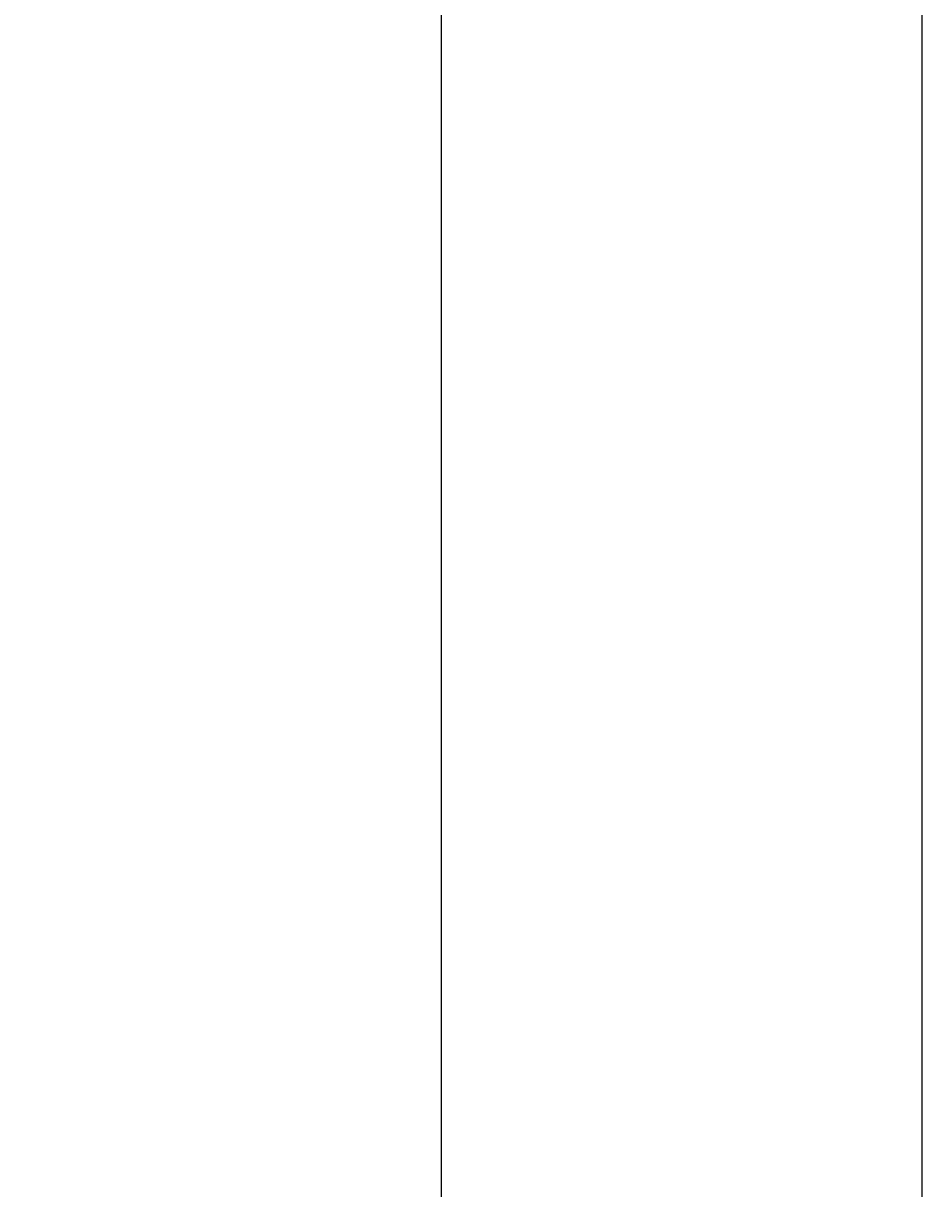
# Model space of a CAD drawing. Units: inches. Extents: x 738 to 1068, y 378 to 757.
# Tile 15 of 41: x 911 to 939, y 399 to 435. Entities that reach past the tile are written whole.
import ezdxf

# ---------------------------------------------------------------- set-up
doc = ezdxf.new("R2010")
doc.units = ezdxf.units.IN
doc.header["$MEASUREMENT"] = 0
doc.layers.add('A-ANNO-DIMS', color=2, linetype='Continuous', lineweight=18)
doc.styles.get("Standard").update_dxf_attribs({"font": 'arial.ttf'})
doc.dimstyles.get("Standard").update_dxf_attribs({"dimtxt": 0.18, "dimasz": 0.18, "dimexe": 0.18, "dimexo": 0.0625, "dimgap": 0.09, "dimtad": 0, "dimtih": 1, "dimtoh": 1, "dimdec": 4, "dimzin": 0, "dimdsep": 46, "dimtxsty": 'Standard', "dimcen": 0.09, "dimadec": 0, "dimazin": 0, "dimtfac": 1, "dimtdec": 4, "dimtofl": 0, "dimtmove": 0, "dimatfit": 3, "dimfxl": 1, "dimtolj": 1, "dimtzin": 0, "dimarcsym": 0})

# ---------------------------------------------------------------- blocks, each defined once
blk = doc.blocks.new('*D17')
at = {"layer": 'A-ANNO-DIMS', "color": 0, "lineweight": -2, "transparency": 16777216}
for p, q in [((756.324, 415.842), (756.324, 378.239)), ((1050.049, 415.919), (1050.049, 378.239)), ((756.504, 378.419), (902.791, 378.419)), ((1049.869, 378.419), (903.582, 378.419))]:
    blk.add_line(p, q, dxfattribs=at)
at = {"layer": 'A-ANNO-DIMS', "color": 0, "transparency": 16777216}
for points in [[(756.504, 378.449), (756.504, 378.389), (756.324, 378.419)], [(1049.869, 378.449), (1049.869, 378.389), (1050.049, 378.419)]]:
    blk.add_solid(points, dxfattribs=at)
at = {"layer": 'Defpoints', "color": 0, "transparency": 16777216}
for p in [(756.324, 415.904), (1050.049, 415.982), (1050.049, 378.419)]:
    blk.add_point(p, dxfattribs=at)
at = {"layer": 'A-ANNO-DIMS', "color": 0, "transparency": 16777216, "insert": (903.186, 378.419), "char_height": 0.18, "attachment_point": 5}
blk.add_mtext('\\A1;293.7', dxfattribs=at)
blk = doc.blocks.new('*D18')
at = {"layer": 'A-ANNO-DIMS', "color": 0, "lineweight": -2, "transparency": 16777216}
for p, q in [((901.525, 738.375), (1068.179, 738.375)), ((1067.999, 738.195), (1067.999, 569.167)), ((1067.999, 399.775), (1067.999, 568.803)), ((1023.842, 399.595), (1068.179, 399.595))]:
    blk.add_line(p, q, dxfattribs=at)
at = {"layer": 'A-ANNO-DIMS', "color": 0, "transparency": 16777216}
for points in [[(1067.969, 738.195), (1068.029, 738.195), (1067.999, 738.375)], [(1067.969, 399.775), (1068.029, 399.775), (1067.999, 399.595)]]:
    blk.add_solid(points, dxfattribs=at)
at = {"layer": 'Defpoints', "color": 0, "transparency": 16777216}
for p in [(901.462, 738.375), (1067.999, 738.375), (1023.779, 399.595)]:
    blk.add_point(p, dxfattribs=at)
at = {"layer": 'A-ANNO-DIMS', "color": 0, "transparency": 16777216, "insert": (1067.999, 568.985), "char_height": 0.18, "attachment_point": 5}
blk.add_mtext('\\A1;338.8', dxfattribs=at)
blk = doc.blocks.new('*D27')
at = {"layer": 'A-ANNO-DIMS', "color": 0, "lineweight": -2, "transparency": 16777216}
for p, q in [((883.457, 646.923), (883.457, 378.239)), ((923.511, 646.923), (923.511, 378.239)), ((883.637, 378.419), (903.086, 378.419)), ((923.331, 378.419), (903.882, 378.419))]:
    blk.add_line(p, q, dxfattribs=at)
at = {"layer": 'A-ANNO-DIMS', "color": 0, "transparency": 16777216}
for points in [[(883.637, 378.449), (883.637, 378.389), (883.457, 378.419)], [(923.331, 378.449), (923.331, 378.389), (923.511, 378.419)]]:
    blk.add_solid(points, dxfattribs=at)
at = {"layer": 'Defpoints', "color": 0, "transparency": 16777216}
for p in [(883.457, 646.985), (923.511, 646.985), (923.511, 378.419)]:
    blk.add_point(p, dxfattribs=at)
at = {"layer": 'A-ANNO-DIMS', "color": 0, "transparency": 16777216, "insert": (903.484, 378.419), "char_height": 0.18, "attachment_point": 5}
blk.add_mtext('\\A1;40.05', dxfattribs=at)
blk = doc.blocks.new('*D28')
at = {"layer": 'A-ANNO-DIMS', "color": 0, "lineweight": -2, "transparency": 16777216}
for p, q in [((923.511, 646.923), (923.511, 378.239)), ((969.439, 646.923), (969.439, 378.239)), ((923.691, 378.419), (946.078, 378.419)), ((969.259, 378.419), (946.872, 378.419))]:
    blk.add_line(p, q, dxfattribs=at)
at = {"layer": 'A-ANNO-DIMS', "color": 0, "transparency": 16777216}
for points in [[(923.691, 378.449), (923.691, 378.389), (923.511, 378.419)], [(969.259, 378.449), (969.259, 378.389), (969.439, 378.419)]]:
    blk.add_solid(points, dxfattribs=at)
at = {"layer": 'Defpoints', "color": 0, "transparency": 16777216}
for p in [(923.511, 646.985), (969.439, 646.985), (969.439, 378.419)]:
    blk.add_point(p, dxfattribs=at)
at = {"layer": 'A-ANNO-DIMS', "color": 0, "transparency": 16777216, "insert": (946.475, 378.419), "char_height": 0.18, "attachment_point": 5}
blk.add_mtext('\\A1;45.93', dxfattribs=at)
blk = doc.blocks.new('*D39')
at = {"layer": 'A-ANNO-DIMS', "color": 0, "lineweight": -2, "transparency": 16777216}
for p, q in [((887.04, 581.418), (887.04, 378.239)), ((938.455, 581.418), (938.455, 378.239)), ((887.22, 378.419), (912.371, 378.419)), ((938.275, 378.419), (913.124, 378.419))]:
    blk.add_line(p, q, dxfattribs=at)
at = {"layer": 'A-ANNO-DIMS', "color": 0, "transparency": 16777216}
for points in [[(887.22, 378.449), (887.22, 378.389), (887.04, 378.419)], [(938.275, 378.449), (938.275, 378.389), (938.455, 378.419)]]:
    blk.add_solid(points, dxfattribs=at)
at = {"layer": 'Defpoints', "color": 0, "transparency": 16777216}
for p in [(887.04, 581.481), (938.455, 581.481), (938.455, 378.419)]:
    blk.add_point(p, dxfattribs=at)
at = {"layer": 'A-ANNO-DIMS', "color": 0, "transparency": 16777216, "insert": (912.748, 378.419), "char_height": 0.18, "attachment_point": 5}
blk.add_mtext('\\A1;51.41', dxfattribs=at)

msp = doc.modelspace()

# ---------------------------------------------------------------- dimensions: what is measured, and where the dimension line sits
at = {"layer": 'A-ANNO-DIMS'}
dim = msp.add_linear_dim(base=(1067.9992, 738.3751), p1=(1023.779, 399.5952), p2=(901.4622, 738.3751), angle=90, dimstyle='Standard', override={"dimdec": 1, "dimlfac": 1, "dimrnd": 0, "dimzin": 0, "dimdsep": 46, "dimlunit": 2}, dxfattribs=at)
dim.commit()
dim.dimension.update_dxf_attribs({"geometry": '*D18', "text_midpoint": (1067.9992, 568.9851)})
for base, p1, p2, override, picture, middle in [((923.5105, 378.4191), (883.4574, 646.9853), (923.5105, 646.9853), {"dimdec": 2, "dimlfac": 1, "dimrnd": 0, "dimzin": 0, "dimdsep": 46, "dimlunit": 2}, '*D27', (903.484, 378.4191)), ((969.4395, 378.4191), (923.5105, 646.9853), (969.4395, 646.9853), {"dimdec": 2, "dimlfac": 1, "dimrnd": 0, "dimzin": 0, "dimdsep": 46, "dimlunit": 2}, '*D28', (946.475, 378.4191)), ((938.455, 378.4191), (887.0404, 581.4808), (938.455, 581.4808), {"dimdec": 2, "dimlfac": 1, "dimrnd": 0, "dimzin": 0, "dimdsep": 46, "dimlunit": 2}, '*D39', (912.7477, 378.4191)), ((1050.0492, 378.4191), (756.3236, 415.904), (1050.0492, 415.982), {"dimdec": 1, "dimlfac": 1, "dimrnd": 0, "dimzin": 0, "dimdsep": 46, "dimlunit": 2}, '*D17', (903.1864, 378.4191))]:
    dim = msp.add_linear_dim(base=base, p1=p1, p2=p2, dimstyle='Standard', override=override, dxfattribs=at)
    dim.commit()
    dim.dimension.update_dxf_attribs({"geometry": picture, "text_midpoint": middle})

doc.saveas('drawing.dxf')
